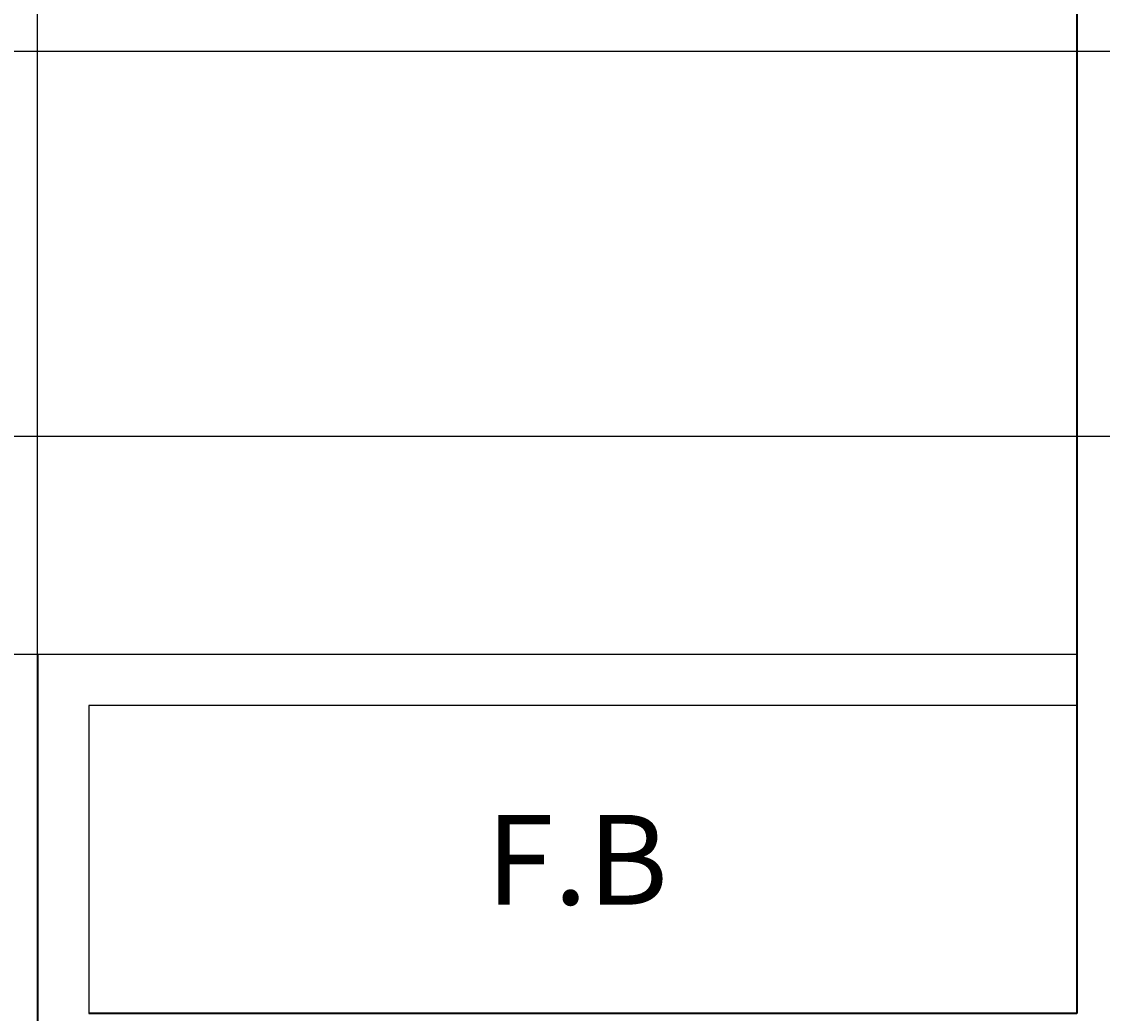
# Model space of a CAD drawing. Units: feet. Extents: x 105 to 1094, y -88 to 588.
# Tile 23 of 59: x 149 to 234, y 396 to 473. Entities that reach past the tile are written whole.
import ezdxf

# ---------------------------------------------------------------- set-up
doc = ezdxf.new("R2010")
doc.units = ezdxf.units.FT
doc.header["$MEASUREMENT"] = 0
for name, color, linetype, lineweight in [('A-ANNO-DIMS', 2, 'Continuous', 18), ('A-ANNO-TEXT', 7, 'Continuous', 18), ('A-FLOR-PROJ', 8, 'Continuous', 25), ('A-WALL', 7, 'Continuous', 35)]:
    doc.layers.add(name, color=color, linetype=linetype, lineweight=lineweight)
doc.styles.get("Standard").update_dxf_attribs({"font": 'arial.ttf'})
doc.dimstyles.get("Standard").update_dxf_attribs({"dimtxt": 0.18, "dimasz": 0.18, "dimexe": 0.18, "dimexo": 0.0625, "dimgap": 0.09, "dimtad": 0, "dimtih": 1, "dimtoh": 1, "dimdec": 4, "dimzin": 0, "dimdsep": 46, "dimtxsty": 'Standard', "dimcen": 0.09, "dimadec": 0, "dimazin": 0, "dimtfac": 1, "dimtdec": 4, "dimtofl": 0, "dimtmove": 0, "dimatfit": 3, "dimfxl": 1, "dimtolj": 1, "dimtzin": 0, "dimarcsym": 0})

# ---------------------------------------------------------------- blocks, each defined once
blk = doc.blocks.new('*D21')
at = {"layer": 'A-ANNO-DIMS', "color": 0, "lineweight": -2, "transparency": 16777216}
for p, q in [((849.626, 543.081), (105.458, 543.081)), ((105.638, 542.901), (105.638, 250.263)), ((105.638, -42.739), (105.638, 249.899)), ((849.626, -42.919), (105.458, -42.919))]:
    blk.add_line(p, q, dxfattribs=at)
at = {"layer": 'A-ANNO-DIMS', "color": 0, "transparency": 16777216}
for points in [[(105.608, 542.901), (105.668, 542.901), (105.638, 543.081)], [(105.608, -42.739), (105.668, -42.739), (105.638, -42.919)]]:
    blk.add_solid(points, dxfattribs=at)
at = {"layer": 'Defpoints', "color": 0, "transparency": 16777216}
for p in [(105.638, 543.081), (849.688, 543.081), (849.688, -42.919)]:
    blk.add_point(p, dxfattribs=at)
at = {"layer": 'A-ANNO-DIMS', "color": 0, "transparency": 16777216, "insert": (105.638, 250.081), "char_height": 0.18, "attachment_point": 5}
blk.add_mtext('\\A1;586', dxfattribs=at)
blk = doc.blocks.new('*D22')
at = {"layer": 'A-ANNO-DIMS', "color": 0, "lineweight": -2, "transparency": 16777216}
for p, q in [((150.688, 424.144), (150.688, 588.311)), ((150.868, 588.131), (190.987, 588.131)), ((231.508, 588.131), (191.39, 588.131)), ((231.688, 543.144), (231.688, 588.311))]:
    blk.add_line(p, q, dxfattribs=at)
at = {"layer": 'A-ANNO-DIMS', "color": 0, "transparency": 16777216}
for points in [[(150.868, 588.161), (150.868, 588.101), (150.688, 588.131)], [(231.508, 588.161), (231.508, 588.101), (231.688, 588.131)]]:
    blk.add_solid(points, dxfattribs=at)
at = {"layer": 'Defpoints', "color": 0, "transparency": 16777216}
for p in [(231.688, 588.131), (231.688, 543.081), (150.688, 424.081)]:
    blk.add_point(p, dxfattribs=at)
at = {"layer": 'A-ANNO-DIMS', "color": 0, "transparency": 16777216, "insert": (191.188, 588.131), "char_height": 0.18, "attachment_point": 5}
blk.add_mtext('\\A1;81', dxfattribs=at)
blk = doc.blocks.new('*D27')
at = {"layer": 'A-ANNO-DIMS', "color": 0, "lineweight": -2, "transparency": 16777216}
for p, q in [((231.626, 543.081), (105.458, 543.081)), ((105.638, 542.901), (105.638, 483.763)), ((105.638, 424.261), (105.638, 483.399)), ((150.626, 424.081), (105.458, 424.081))]:
    blk.add_line(p, q, dxfattribs=at)
at = {"layer": 'A-ANNO-DIMS', "color": 0, "transparency": 16777216}
for points in [[(105.608, 542.901), (105.668, 542.901), (105.638, 543.081)], [(105.608, 424.261), (105.668, 424.261), (105.638, 424.081)]]:
    blk.add_solid(points, dxfattribs=at)
at = {"layer": 'Defpoints', "color": 0, "transparency": 16777216}
for p in [(105.638, 543.081), (231.688, 543.081), (150.688, 424.081)]:
    blk.add_point(p, dxfattribs=at)
at = {"layer": 'A-ANNO-DIMS', "color": 0, "transparency": 16777216, "insert": (105.638, 483.581), "char_height": 0.18, "attachment_point": 5}
blk.add_mtext('\\A1;119', dxfattribs=at)
blk = doc.blocks.new('*D28')
at = {"layer": 'A-ANNO-DIMS', "color": 0, "lineweight": -2, "transparency": 16777216}
for p, q in [((150.626, 424.081), (105.458, 424.081)), ((105.638, 423.901), (105.638, 350.263)), ((105.638, 276.261), (105.638, 349.899)), ((150.626, 276.081), (105.458, 276.081))]:
    blk.add_line(p, q, dxfattribs=at)
at = {"layer": 'A-ANNO-DIMS', "color": 0, "transparency": 16777216}
for points in [[(105.608, 423.901), (105.668, 423.901), (105.638, 424.081)], [(105.608, 276.261), (105.668, 276.261), (105.638, 276.081)]]:
    blk.add_solid(points, dxfattribs=at)
at = {"layer": 'Defpoints', "color": 0, "transparency": 16777216}
for p in [(105.638, 424.081), (150.688, 424.081), (150.688, 276.081)]:
    blk.add_point(p, dxfattribs=at)
at = {"layer": 'A-ANNO-DIMS', "color": 0, "transparency": 16777216, "insert": (105.638, 350.081), "char_height": 0.18, "attachment_point": 5}
blk.add_mtext('\\A1;148', dxfattribs=at)
blk = doc.blocks.new('*D32')
at = {"layer": 'A-ANNO-DIMS', "color": 0, "lineweight": -2, "transparency": 16777216}
for p, q in [((646.626, 471.081), (105.458, 471.081)), ((105.638, 470.901), (105.638, 456.263)), ((105.638, 441.261), (105.638, 455.899)), ((646.626, 441.081), (105.458, 441.081))]:
    blk.add_line(p, q, dxfattribs=at)
at = {"layer": 'A-ANNO-DIMS', "color": 0, "transparency": 16777216}
for points in [[(105.608, 470.901), (105.668, 470.901), (105.638, 471.081)], [(105.608, 441.261), (105.668, 441.261), (105.638, 441.081)]]:
    blk.add_solid(points, dxfattribs=at)
at = {"layer": 'Defpoints', "color": 0, "transparency": 16777216}
for p in [(105.638, 471.081), (646.688, 471.081), (646.688, 441.081)]:
    blk.add_point(p, dxfattribs=at)
at = {"layer": 'A-ANNO-DIMS', "color": 0, "transparency": 16777216, "insert": (105.638, 456.081), "char_height": 0.18, "attachment_point": 5}
blk.add_mtext('\\A1;30', dxfattribs=at)
blk = doc.blocks.new('*D38')
at = {"layer": 'A-ANNO-DIMS', "color": 0, "lineweight": -2, "transparency": 16777216}
for p, q in [((150.688, 224.144), (150.688, 588.311)), ((150.868, 588.131), (222.408, 588.131)), ((294.508, 588.131), (222.968, 588.131)), ((294.688, 224.144), (294.688, 588.311))]:
    blk.add_line(p, q, dxfattribs=at)
at = {"layer": 'A-ANNO-DIMS', "color": 0, "transparency": 16777216}
for points in [[(150.868, 588.161), (150.868, 588.101), (150.688, 588.131)], [(294.508, 588.161), (294.508, 588.101), (294.688, 588.131)]]:
    blk.add_solid(points, dxfattribs=at)
at = {"layer": 'Defpoints', "color": 0, "transparency": 16777216}
for p in [(294.688, 588.131), (150.688, 224.081), (294.688, 224.081)]:
    blk.add_point(p, dxfattribs=at)
at = {"layer": 'A-ANNO-DIMS', "color": 0, "transparency": 16777216, "insert": (222.688, 588.131), "char_height": 0.18, "attachment_point": 5}
blk.add_mtext('\\A1;144', dxfattribs=at)

msp = doc.modelspace()

# ---------------------------------------------------------------- linework, layer by layer
at = {"layer": 'A-FLOR-PROJ'}
for p, q in [((231.6883, 424.0812), (150.6883, 424.0812)), ((150.6883, 424.0812), (150.6883, 394.0812)), ((231.6883, 420.0812), (154.6883, 420.0812)), ((154.6883, 420.0812), (154.6883, 396.0812))]:
    msp.add_line(p, q, dxfattribs=at)
at = {"layer": 'A-WALL'}
for p, q in [((231.6883, 513.0812), (231.6883, 396.0812)), ((231.6883, 396.0812), (154.6883, 396.0812))]:
    msp.add_line(p, q, dxfattribs=at)

# ---------------------------------------------------------------- texts
at = {"layer": 'A-ANNO-TEXT', "insert": (241.9039, 411.5608), "char_height": 7, "attachment_point": 3}
msp.add_mtext_dynamic_manual_height_columns('\\pxqc;F.B ', width=98.34246, gutter_width=1, heights=[0], dxfattribs=at)

# ---------------------------------------------------------------- dimensions: what is measured, and where the dimension line sits
at = {"layer": 'A-ANNO-DIMS'}
for base, p1, p2, picture, middle in [((231.6883, 588.1312), (150.6883, 424.0812), (231.6883, 543.0812), '*D22', (191.1883, 588.1312)), ((294.6883, 588.1312), (150.6883, 224.0812), (294.6883, 224.0812), '*D38', (222.6883, 588.1312))]:
    dim = msp.add_linear_dim(base=base, p1=p1, p2=p2, dimstyle='Standard', override={"dimdec": 0, "dimlfac": 1, "dimrnd": 0, "dimzin": 0, "dimdsep": 46, "dimlunit": 2}, dxfattribs=at)
    dim.commit()
    dim.dimension.update_dxf_attribs({"geometry": picture, "text_midpoint": middle})
for base, p1, p2, picture, middle in [((105.6383, 543.0812), (849.6883, -42.9188), (849.6883, 543.0812), '*D21', (105.6383, 250.0812)), ((105.6383, 543.0812), (150.6883, 424.0812), (231.6883, 543.0812), '*D27', (105.6383, 483.5812)), ((105.6383, 471.0812), (646.6883, 441.0812), (646.6883, 471.0812), '*D32', (105.6383, 456.0812)), ((105.6383, 424.0812), (150.6883, 276.0812), (150.6883, 424.0812), '*D28', (105.6383, 350.0812))]:
    dim = msp.add_linear_dim(base=base, p1=p1, p2=p2, angle=90, dimstyle='Standard', override={"dimdec": 0, "dimlfac": 1, "dimrnd": 0, "dimzin": 0, "dimdsep": 46, "dimlunit": 2}, dxfattribs=at)
    dim.commit()
    dim.dimension.update_dxf_attribs({"geometry": picture, "text_midpoint": middle})

doc.saveas('drawing.dxf')
